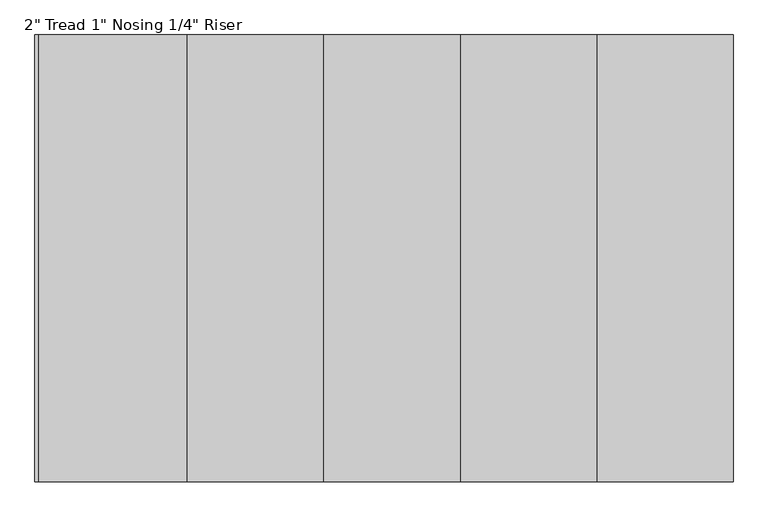
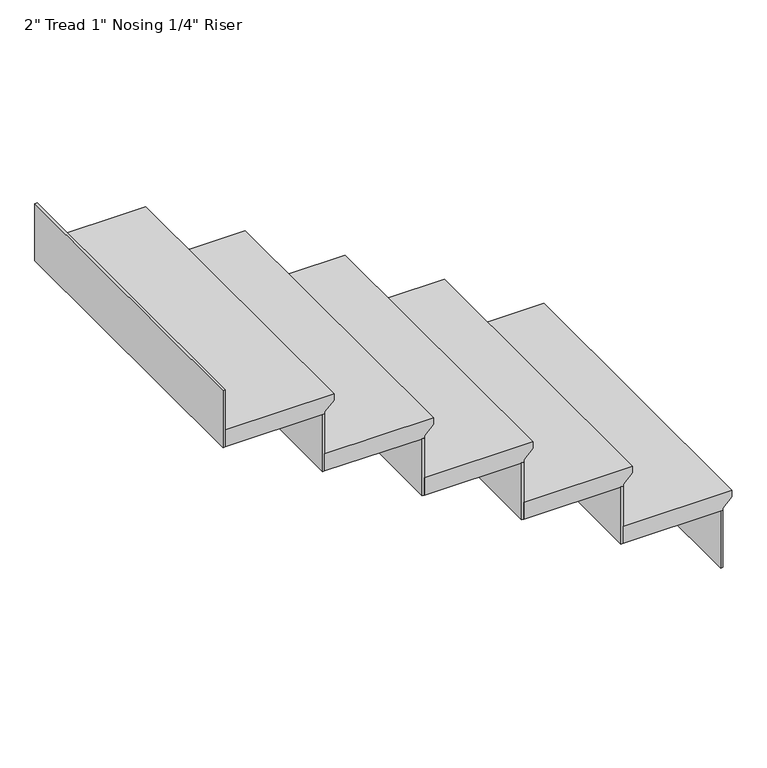
"""IFC4 building model written with IfcOpenShell, lengths in millimetres: stair flight geometry."""

from ifc_helpers import new_model, si_unit, frame, origin, place, context, project, spatial, polyline, outline, extrude, source, transform, mapped, element, save


def stair_flight_16b82674(model_context):
    return source(origin(), model_context, "Body", "SweptSolid", [
        extrude(outline(polyline([(5249.3333333, 2644.5430349), (5249.3333333, 2339.7430349), (5198.5333333, 2339.7430349), (5198.5333333, 2619.1430349), (5204.8833333, 2619.1430349), (5230.2833333, 2644.5430349), (5249.3333333, 2644.5430349)])), frame((0.0, 2083.4555142, 0.0), z_axis=(0.0, 1.0, 0.0), x_axis=(0.0, 0.0, 1.0)), (0.0, 0.0, 1.0), 914.4),
        extrude(outline(polyline([(2612.7930349, 2997.8555142), (2619.1430349, 2997.8555142), (2619.1430349, 2083.4555142), (2612.7930349, 2083.4555142), (2612.7930349, 2997.8555142)])), frame((0.0, 0.0, 5029.2), z_axis=(0.0, 0.0, 1.0), x_axis=(1.0, 0.0, 0.0)), (0.0, 0.0, 1.0), 169.3333333),
        extrude(outline(polyline([(2333.3930349, 2997.8555142), (2339.7430349, 2997.8555142), (2339.7430349, 2083.4555142), (2333.3930349, 2083.4555142), (2333.3930349, 2997.8555142)])), frame((0.0, 0.0, 5198.5333333), z_axis=(0.0, 0.0, 1.0), x_axis=(1.0, 0.0, 0.0)), (0.0, 0.0, 1.0), 169.3333333),
        extrude(outline(polyline([(5418.6666667, 2365.1430349), (5418.6666667, 2060.3430349), (5367.8666667, 2060.3430349), (5367.8666667, 2339.7430349), (5374.2166667, 2339.7430349), (5399.6166667, 2365.1430349), (5418.6666667, 2365.1430349)])), frame((0.0, 2083.4555142, 0.0), z_axis=(0.0, 1.0, 0.0), x_axis=(0.0, 0.0, 1.0)), (0.0, 0.0, 1.0), 914.4),
        extrude(outline(polyline([(2053.9930349, 2997.8555142), (2060.3430349, 2997.8555142), (2060.3430349, 2083.4555142), (2053.9930349, 2083.4555142), (2053.9930349, 2997.8555142)])), frame((0.0, 0.0, 5367.8666667), z_axis=(0.0, 0.0, 1.0), x_axis=(1.0, 0.0, 0.0)), (0.0, 0.0, 1.0), 169.3333333),
        extrude(outline(polyline([(5588.0, 2085.7430349), (5588.0, 1780.9430349), (5537.2, 1780.9430349), (5537.2, 2060.3430349), (5543.55, 2060.3430349), (5568.95, 2085.7430349), (5588.0, 2085.7430349)])), frame((0.0, 2083.4555142, 0.0), z_axis=(0.0, 1.0, 0.0), x_axis=(0.0, 0.0, 1.0)), (0.0, 0.0, 1.0), 914.4),
        extrude(outline(polyline([(1774.5930349, 2997.8555142), (1780.9430349, 2997.8555142), (1780.9430349, 2083.4555142), (1774.5930349, 2083.4555142), (1774.5930349, 2997.8555142)])), frame((0.0, 0.0, 5537.2), z_axis=(0.0, 0.0, 1.0), x_axis=(1.0, 0.0, 0.0)), (0.0, 0.0, 1.0), 169.3333333),
        extrude(outline(polyline([(5757.3333333, 1806.3430349), (5757.3333333, 1501.5430349), (5706.5333333, 1501.5430349), (5706.5333333, 1780.9430349), (5712.8833333, 1780.9430349), (5738.2833333, 1806.3430349), (5757.3333333, 1806.3430349)])), frame((0.0, 2083.4555142, 0.0), z_axis=(0.0, 1.0, 0.0), x_axis=(0.0, 0.0, 1.0)), (0.0, 0.0, 1.0), 914.4),
        extrude(outline(polyline([(1495.1930349, 2997.8555142), (1501.5430349, 2997.8555142), (1501.5430349, 2083.4555142), (1495.1930349, 2083.4555142), (1495.1930349, 2997.8555142)])), frame((0.0, 0.0, 5706.5333333), z_axis=(0.0, 0.0, 1.0), x_axis=(1.0, 0.0, 0.0)), (0.0, 0.0, 1.0), 169.3333333),
        extrude(outline(polyline([(1215.7930349, 2997.8555142), (1222.1430349, 2997.8555142), (1222.1430349, 2083.4555142), (1215.7930349, 2083.4555142), (1215.7930349, 2997.8555142)])), frame((0.0, 0.0, 5875.8666667), z_axis=(0.0, 0.0, 1.0), x_axis=(1.0, 0.0, 0.0)), (0.0, 0.0, 1.0), 169.3333333),
        extrude(outline(polyline([(5926.6666667, 1526.9430349), (5926.6666667, 1222.1430349), (5875.8666667, 1222.1430349), (5875.8666667, 1501.5430349), (5882.2166667, 1501.5430349), (5907.6166667, 1526.9430349), (5926.6666667, 1526.9430349)])), frame((0.0, 2083.4555142, 0.0), z_axis=(0.0, 1.0, 0.0), x_axis=(0.0, 0.0, 1.0)), (0.0, 0.0, 1.0), 914.4),
    ])


if __name__ == "__main__":
    model = new_model("IFC4")
    model_context = context("Model", 3, world=origin())
    ifc_project = project(units=[si_unit("LENGTHUNIT", "METRE", prefix="MILLI")], contexts=[model_context])
    site = spatial("IfcSite", under=ifc_project)
    building = spatial("IfcBuilding", under=site)
    placement = place(None, origin())
    stair_flight_shape = stair_flight_16b82674(model_context)
    element("IfcStairFlight", 1, ObjectType="2\" Tread 1\" Nosing 1/4\" Riser", at=placement, inside=building, context=model_context, shape_type="MappedRepresentation", body=[
        mapped(stair_flight_shape, transform((0.0, 0.0, 0.0), x_axis=(1.0, 0.0, 0.0), y_axis=(0.0, 1.0, 0.0), z_axis=(0.0, 0.0, 1.0))),
    ])
    save(model, "model.ifc")
